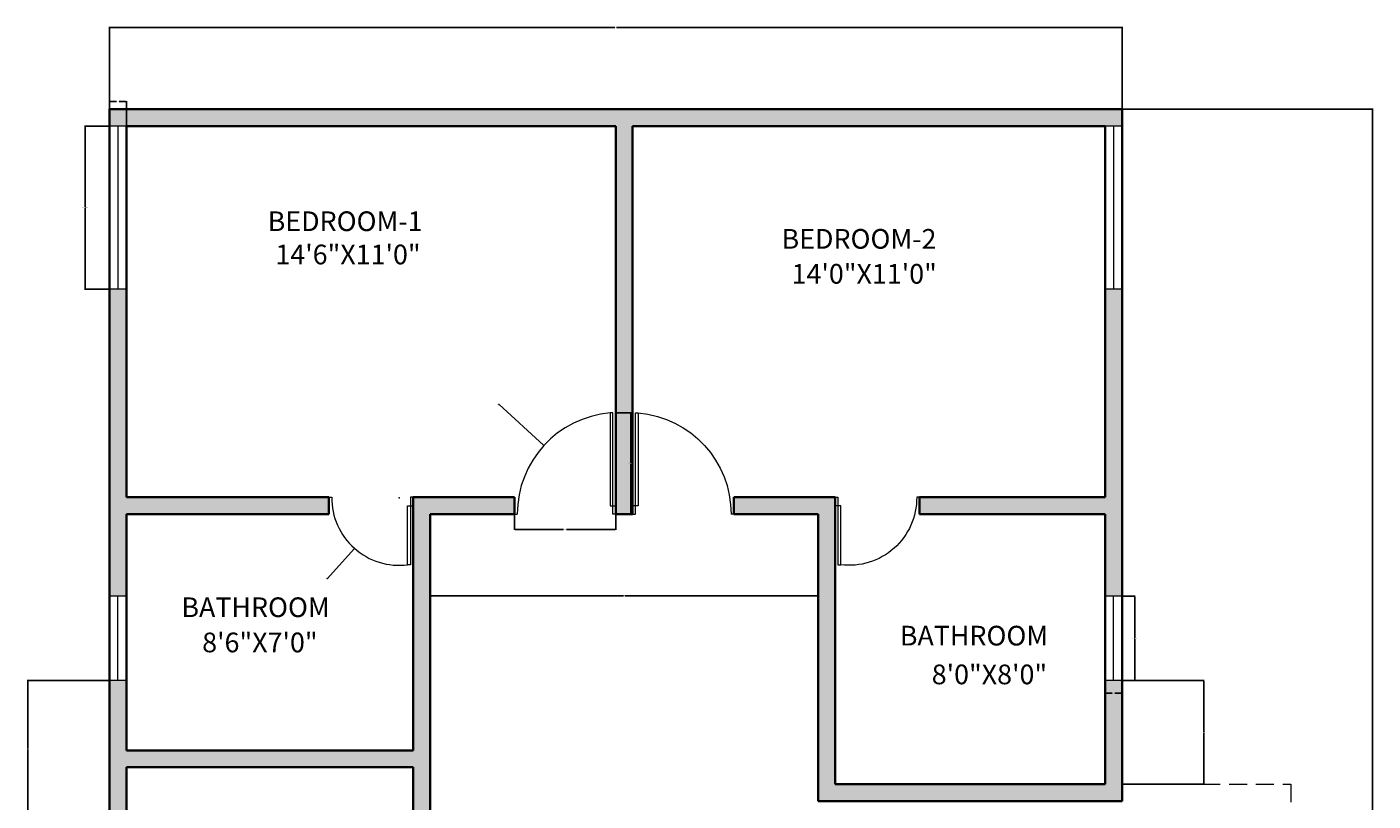
# Model space of a CAD drawing. Units: inches. Extents: x 2886 to 3365, y 1372 to 2008.
# Tile 2 of 2: x 2886 to 3365, y 1733 to 2008. Entities that reach past the tile are written whole.
import ezdxf

# ---------------------------------------------------------------- set-up
doc = ezdxf.new("R2010")
doc.units = ezdxf.units.IN
doc.linetypes.add('DASHED2', pattern=[9.525, 6.35, -3.175])
for name, color, linetype, lineweight in [('A-ANNO-DIMS', 2, 'Continuous', 18), ('A-AREA-IDEN', 50, 'Continuous', 18), ('A-DOOR', 230, 'Continuous', 18), ('A-FLOR-OVHD', 7, 'DASHED2', 18), ('A-GLAZ', 7, 'Continuous', 18), ('A-WALL', 7, 'Continuous', 35)]:
    doc.layers.add(name, color=color, linetype=linetype, lineweight=lineweight)
doc.layers.add('A-WALL-PATT', color=18, linetype='Continuous', lineweight=13, true_color=0x000000)
doc.styles.get("Standard").update_dxf_attribs({"font": 'arial.ttf'})
doc.dimstyles.get("Standard").update_dxf_attribs({"dimtxt": 0.18, "dimasz": 0.18, "dimexe": 0.18, "dimexo": 0.0625, "dimgap": 0.09, "dimtad": 0, "dimtih": 1, "dimtoh": 1, "dimdec": 4, "dimzin": 0, "dimdsep": 46, "dimtxsty": 'Standard', "dimcen": 0.09, "dimadec": 0, "dimazin": 0, "dimtfac": 1, "dimtdec": 4, "dimtofl": 0, "dimtmove": 0, "dimatfit": 3, "dimfxl": 1, "dimtolj": 1, "dimtzin": 0, "dimarcsym": 0})

# ---------------------------------------------------------------- blocks, each defined once
blk = doc.blocks.new('DOOR-SWING-30IN')
for p, q in [((0, 24.19), (1, 24.19)), ((30, 24.19), (29, 24.19)), ((29, 24.19), (29, 0.19)), ((28, 0.19), (28, 21.19)), ((28, 21.19), (30, 21.19)), ((29, 0.19), (28, 0.19))]:
    blk.add_line(p, q)
blk.add_arc((25, 24), 24, 179.5504, 277.1825)
blk = doc.blocks.new('DOOR-SWING-36IN')
for p, q in [((35, 36), (34, 36)), ((34, 36), (34, 3)), ((35, 0), (35, 36)), ((0, 0), (1, 0)), ((34, 3), (36, 3)), ((36, 0), (35, 0))]:
    blk.add_line(p, q)
blk.add_arc((37, 0.13), 36, 94.7798, 180.1993)
blk = doc.blocks.new('WIN-30IN')
for p, q in [((6, 30), (0, 30)), ((3, 0), (3, 30)), ((6, 0), (0, 0))]:
    blk.add_line(p, q)
blk = doc.blocks.new('WIN-58IN')
for p, q in [((6, 58), (0, 58)), ((3, 58), (3, 0)), ((6, 0), (0, 0))]:
    blk.add_line(p, q)
blk = doc.blocks.new('*D7')
at = {"layer": 'A-ANNO-DIMS', "color": 0, "lineweight": -2, "transparency": 16777216}
for p, q in [((3095.42, 1870.96), (3100.94, 1870.96)), ((3100.76, 1870.78), (3100.76, 1853.15)), ((3100.76, 1835.14), (3100.76, 1852.78)), ((3095.42, 1834.96), (3100.94, 1834.96))]:
    blk.add_line(p, q, dxfattribs=at)
at = {"layer": 'A-ANNO-DIMS', "color": 0, "transparency": 16777216}
for points in [[(3100.73, 1870.78), (3100.79, 1870.78), (3100.76, 1870.96)], [(3100.73, 1835.14), (3100.79, 1835.14), (3100.76, 1834.96)]]:
    blk.add_solid(points, dxfattribs=at)
at = {"layer": 'Defpoints', "color": 0, "transparency": 16777216}
for p in [(3095.36, 1870.96), (3100.76, 1870.96), (3095.36, 1834.96)]:
    blk.add_point(p, dxfattribs=at)
at = {"layer": 'A-ANNO-DIMS', "color": 0, "transparency": 16777216, "insert": (3100.76, 1852.96), "char_height": 0.18, "attachment_point": 5}
blk.add_mtext('\\A1;DOOR 36 TYP.', dxfattribs=at)
blk = doc.blocks.new('*D8')
at = {"layer": 'A-ANNO-DIMS', "color": 0, "lineweight": -2, "transparency": 16777216}
for p, q in [((3059.36, 1834.9), (3059.36, 1829.38)), ((3095.36, 1834.9), (3095.36, 1829.38)), ((3059.54, 1829.56), (3076.83, 1829.56)), ((3095.18, 1829.56), (3077.89, 1829.56))]:
    blk.add_line(p, q, dxfattribs=at)
at = {"layer": 'A-ANNO-DIMS', "color": 0, "transparency": 16777216}
for points in [[(3059.54, 1829.59), (3059.54, 1829.53), (3059.36, 1829.56)], [(3095.18, 1829.59), (3095.18, 1829.53), (3095.36, 1829.56)]]:
    blk.add_solid(points, dxfattribs=at)
at = {"layer": 'Defpoints', "color": 0, "transparency": 16777216}
for p in [(3059.36, 1834.96), (3095.36, 1834.96), (3095.36, 1829.56)]:
    blk.add_point(p, dxfattribs=at)
at = {"layer": 'A-ANNO-DIMS', "color": 0, "transparency": 16777216, "insert": (3077.36, 1829.56), "char_height": 0.18, "attachment_point": 5}
blk.add_mtext('\\A1;36 TYP.', dxfattribs=at)
blk = doc.blocks.new('*D9')
at = {"layer": 'A-ANNO-DIMS', "color": 0, "lineweight": -2, "transparency": 16777216}
for p, q in [((3275.42, 1805.81), (3280.04, 1805.81)), ((3279.86, 1805.63), (3279.86, 1790.99)), ((3279.86, 1775.99), (3279.86, 1790.63)), ((3275.42, 1775.81), (3280.04, 1775.81))]:
    blk.add_line(p, q, dxfattribs=at)
at = {"layer": 'A-ANNO-DIMS', "color": 0, "transparency": 16777216}
for points in [[(3279.83, 1805.63), (3279.89, 1805.63), (3279.86, 1805.81)], [(3279.83, 1775.99), (3279.89, 1775.99), (3279.86, 1775.81)]]:
    blk.add_solid(points, dxfattribs=at)
at = {"layer": 'Defpoints', "color": 0, "transparency": 16777216}
for p in [(3275.36, 1805.81), (3279.86, 1805.81), (3275.36, 1775.81)]:
    blk.add_point(p, dxfattribs=at)
at = {"layer": 'A-ANNO-DIMS', "color": 0, "transparency": 16777216, "insert": (3279.86, 1790.81), "char_height": 0.18, "attachment_point": 5}
blk.add_mtext('\\A1;WINDOW 30 TYP.', dxfattribs=at)
blk = doc.blocks.new('*D10')
at = {"layer": 'A-ANNO-DIMS', "color": 0, "lineweight": -2, "transparency": 16777216}
for p, q in [((3269.36, 1775.75), (3269.36, 1771.13)), ((3275.36, 1775.75), (3275.36, 1771.13)), ((3269.54, 1771.31), (3271.9, 1771.31)), ((3275.18, 1771.31), (3272.82, 1771.31))]:
    blk.add_line(p, q, dxfattribs=at)
at = {"layer": 'A-ANNO-DIMS', "color": 0, "transparency": 16777216}
for points in [[(3269.54, 1771.34), (3269.54, 1771.28), (3269.36, 1771.31)], [(3275.18, 1771.34), (3275.18, 1771.28), (3275.36, 1771.31)]]:
    blk.add_solid(points, dxfattribs=at)
at = {"layer": 'Defpoints', "color": 0, "transparency": 16777216}
for p in [(3269.36, 1775.81), (3275.36, 1775.81), (3275.36, 1771.31)]:
    blk.add_point(p, dxfattribs=at)
at = {"layer": 'A-ANNO-DIMS', "color": 0, "transparency": 16777216, "insert": (3272.36, 1771.31), "char_height": 0.18, "attachment_point": 5}
blk.add_mtext('\\A1;6 TYP.', dxfattribs=at)
blk = doc.blocks.new('*D11')
at = {"layer": 'A-ANNO-DIMS', "color": 0, "lineweight": -2, "transparency": 16777216}
for p, q in [((2915.29, 1972.96), (2906.48, 1972.96)), ((2906.66, 1972.78), (2906.66, 1944.15)), ((2906.66, 1915.14), (2906.66, 1943.78)), ((2915.29, 1914.96), (2906.48, 1914.96))]:
    blk.add_line(p, q, dxfattribs=at)
at = {"layer": 'A-ANNO-DIMS', "color": 0, "transparency": 16777216}
for points in [[(2906.63, 1972.78), (2906.69, 1972.78), (2906.66, 1972.96)], [(2906.63, 1915.14), (2906.69, 1915.14), (2906.66, 1914.96)]]:
    blk.add_solid(points, dxfattribs=at)
at = {"layer": 'Defpoints', "color": 0, "transparency": 16777216}
for p in [(2906.66, 1972.96), (2915.36, 1972.96), (2915.36, 1914.96)]:
    blk.add_point(p, dxfattribs=at)
at = {"layer": 'A-ANNO-DIMS', "color": 0, "transparency": 16777216, "insert": (2906.66, 1943.96), "char_height": 0.18, "attachment_point": 5}
blk.add_mtext('\\A1;WINDOW 58 TYP.', dxfattribs=at)
blk = doc.blocks.new('*D12')
at = {"layer": 'A-ANNO-DIMS', "color": 0, "lineweight": -2, "transparency": 16777216}
for p, q in [((2915.36, 1973.02), (2915.36, 1981.84)), ((2915.54, 1981.66), (2917.9, 1981.66)), ((2921.18, 1981.66), (2918.82, 1981.66)), ((2921.36, 1973.02), (2921.36, 1981.84))]:
    blk.add_line(p, q, dxfattribs=at)
at = {"layer": 'A-ANNO-DIMS', "color": 0, "transparency": 16777216}
for points in [[(2915.54, 1981.69), (2915.54, 1981.63), (2915.36, 1981.66)], [(2921.18, 1981.69), (2921.18, 1981.63), (2921.36, 1981.66)]]:
    blk.add_solid(points, dxfattribs=at)
at = {"layer": 'Defpoints', "color": 0, "transparency": 16777216}
for p in [(2921.36, 1981.66), (2915.36, 1972.96), (2921.36, 1972.96)]:
    blk.add_point(p, dxfattribs=at)
at = {"layer": 'A-ANNO-DIMS', "color": 0, "transparency": 16777216, "insert": (2918.36, 1981.66), "char_height": 0.18, "attachment_point": 5}
blk.add_mtext('\\A1;6 TYP.', dxfattribs=at)
blk = doc.blocks.new('*D14')
at = {"layer": 'A-ANNO-DIMS', "color": 0, "lineweight": -2, "transparency": 16777216}
for p, q in [((3275.42, 1978.96), (3364.59, 1978.96)), ((3364.41, 1978.78), (3364.41, 1690.14)), ((3364.41, 1401.14), (3364.41, 1689.78)), ((3275.42, 1400.96), (3364.59, 1400.96))]:
    blk.add_line(p, q, dxfattribs=at)
at = {"layer": 'A-ANNO-DIMS', "color": 0, "transparency": 16777216}
for points in [[(3364.38, 1978.78), (3364.44, 1978.78), (3364.41, 1978.96)], [(3364.38, 1401.14), (3364.44, 1401.14), (3364.41, 1400.96)]]:
    blk.add_solid(points, dxfattribs=at)
at = {"layer": 'Defpoints', "color": 0, "transparency": 16777216}
for p in [(3275.36, 1978.96), (3364.41, 1978.96), (3275.36, 1400.96)]:
    blk.add_point(p, dxfattribs=at)
at = {"layer": 'A-ANNO-DIMS', "color": 0, "transparency": 16777216, "insert": (3364.41, 1689.96), "char_height": 0.18, "attachment_point": 5}
blk.add_mtext('\\A1;578', dxfattribs=at)
blk = doc.blocks.new('*D15')
at = {"layer": 'A-ANNO-DIMS', "color": 0, "lineweight": -2, "transparency": 16777216}
for p, q in [((2915.36, 1979.02), (2915.36, 2008.19)), ((2915.54, 2008.01), (3095.07, 2008.01)), ((3275.18, 2008.01), (3095.65, 2008.01)), ((3275.36, 1979.02), (3275.36, 2008.19))]:
    blk.add_line(p, q, dxfattribs=at)
at = {"layer": 'A-ANNO-DIMS', "color": 0, "transparency": 16777216}
for points in [[(2915.54, 2008.04), (2915.54, 2007.98), (2915.36, 2008.01)], [(3275.18, 2008.04), (3275.18, 2007.98), (3275.36, 2008.01)]]:
    blk.add_solid(points, dxfattribs=at)
at = {"layer": 'Defpoints', "color": 0, "transparency": 16777216}
for p in [(3275.36, 2008.01), (2915.36, 1978.96), (3275.36, 1978.96)]:
    blk.add_point(p, dxfattribs=at)
at = {"layer": 'A-ANNO-DIMS', "color": 0, "transparency": 16777216, "insert": (3095.36, 2008.01), "char_height": 0.18, "attachment_point": 5}
blk.add_mtext('\\A1;360', dxfattribs=at)
blk = doc.blocks.new('*D20')
at = {"layer": 'A-ANNO-DIMS', "color": 0, "lineweight": -2, "transparency": 16777216}
for p, q in [((2915.29, 1775.81), (2886.13, 1775.81)), ((2886.31, 1775.63), (2886.31, 1751.69)), ((2886.31, 1727.38), (2886.31, 1751.32)), ((2915.29, 1727.2), (2886.13, 1727.2))]:
    blk.add_line(p, q, dxfattribs=at)
at = {"layer": 'A-ANNO-DIMS', "color": 0, "transparency": 16777216}
for points in [[(2886.28, 1775.63), (2886.34, 1775.63), (2886.31, 1775.81)], [(2886.28, 1727.38), (2886.34, 1727.38), (2886.31, 1727.2)]]:
    blk.add_solid(points, dxfattribs=at)
at = {"layer": 'Defpoints', "color": 0, "transparency": 16777216}
for p in [(2886.31, 1775.81), (2915.36, 1775.81), (2915.36, 1727.2)]:
    blk.add_point(p, dxfattribs=at)
at = {"layer": 'A-ANNO-DIMS', "color": 0, "transparency": 16777216, "insert": (2886.31, 1751.5), "char_height": 0.18, "attachment_point": 5}
blk.add_mtext('\\A1;48.61', dxfattribs=at)
blk = doc.blocks.new('*D23')
at = {"layer": 'A-ANNO-DIMS', "color": 0, "lineweight": -2, "transparency": 16777216}
for p, q in [((3275.42, 1775.81), (3304.59, 1775.81)), ((3304.41, 1775.63), (3304.41, 1757.57)), ((3304.41, 1739.14), (3304.41, 1757.2)), ((3275.42, 1738.96), (3304.59, 1738.96))]:
    blk.add_line(p, q, dxfattribs=at)
at = {"layer": 'A-ANNO-DIMS', "color": 0, "transparency": 16777216}
for points in [[(3304.38, 1775.63), (3304.44, 1775.63), (3304.41, 1775.81)], [(3304.38, 1739.14), (3304.44, 1739.14), (3304.41, 1738.96)]]:
    blk.add_solid(points, dxfattribs=at)
at = {"layer": 'Defpoints', "color": 0, "transparency": 16777216}
for p in [(3275.36, 1775.81), (3275.36, 1738.96), (3304.41, 1738.96)]:
    blk.add_point(p, dxfattribs=at)
at = {"layer": 'A-ANNO-DIMS', "color": 0, "transparency": 16777216, "insert": (3304.41, 1757.39), "char_height": 0.18, "attachment_point": 5}
blk.add_mtext('\\A1;36.85', dxfattribs=at)
blk = doc.blocks.new('*D25')
at = {"layer": 'A-ANNO-DIMS', "color": 0, "lineweight": -2, "transparency": 16777216}
for p, q in [((3029.36, 1834.9), (3029.36, 1805.73)), ((3167.36, 1834.9), (3167.36, 1805.73)), ((3029.54, 1805.91), (3098.08, 1805.91)), ((3167.18, 1805.91), (3098.64, 1805.91))]:
    blk.add_line(p, q, dxfattribs=at)
at = {"layer": 'A-ANNO-DIMS', "color": 0, "transparency": 16777216}
for points in [[(3029.54, 1805.94), (3029.54, 1805.88), (3029.36, 1805.91)], [(3167.18, 1805.94), (3167.18, 1805.88), (3167.36, 1805.91)]]:
    blk.add_solid(points, dxfattribs=at)
at = {"layer": 'Defpoints', "color": 0, "transparency": 16777216}
for p in [(3029.36, 1834.96), (3167.36, 1834.96), (3029.36, 1805.91)]:
    blk.add_point(p, dxfattribs=at)
at = {"layer": 'A-ANNO-DIMS', "color": 0, "transparency": 16777216, "insert": (3098.36, 1805.91), "char_height": 0.18, "attachment_point": 5}
blk.add_mtext('\\A1;138', dxfattribs=at)
blk = doc.blocks.new('*D31')
at = {"layer": 'A-ANNO-DIMS', "color": 0, "lineweight": -2, "transparency": 16777216}
for p, q in [((3053.72, 1874.01), (3053.9, 1874.01)), ((3053.9, 1874.01), (3069.69, 1859.54)), ((3096.27, 1835.09), (3096.45, 1835.09)), ((3096.36, 1835), (3096.36, 1835.18))]:
    blk.add_line(p, q, dxfattribs=at)
at = {"layer": 'A-ANNO-DIMS', "color": 0, "transparency": 16777216}
blk.add_solid([(3069.71, 1859.56), (3069.67, 1859.51), (3069.82, 1859.41)], dxfattribs=at)
at = {"layer": 'Defpoints', "color": 0, "transparency": 16777216}
for p in [(3069.82, 1859.41), (3096.36, 1835.09)]:
    blk.add_point(p, dxfattribs=at)
at = {"layer": 'A-ANNO-DIMS', "color": 0, "transparency": 16777216, "insert": (3053.41, 1874.01), "char_height": 0.18, "attachment_point": 5}
blk.add_mtext('\\A1;R36', dxfattribs=at)
blk = doc.blocks.new('*D32')
at = {"layer": 'A-ANNO-DIMS', "color": 0, "lineweight": -2, "transparency": 16777216}
for p, q in [((3018.27, 1840.77), (3018.45, 1840.77)), ((3018.36, 1840.68), (3018.36, 1840.86)), ((2992.85, 1812.07), (3002.29, 1822.7)), ((2992.67, 1812.07), (2992.85, 1812.07))]:
    blk.add_line(p, q, dxfattribs=at)
at = {"layer": 'A-ANNO-DIMS', "color": 0, "transparency": 16777216}
blk.add_solid([(3002.27, 1822.72), (3002.31, 1822.68), (3002.41, 1822.84)], dxfattribs=at)
at = {"layer": 'Defpoints', "color": 0, "transparency": 16777216}
for p in [(3018.36, 1840.77), (3002.41, 1822.84)]:
    blk.add_point(p, dxfattribs=at)
at = {"layer": 'A-ANNO-DIMS', "color": 0, "transparency": 16777216, "insert": (2992.17, 1812.07), "char_height": 0.18, "attachment_point": 5}
blk.add_mtext('\\A1;3X R24', dxfattribs=at)

msp = doc.modelspace()

# ---------------------------------------------------------------- hatches: boundary and pattern name
at = {"layer": 'A-WALL-PATT'}
h = msp.add_hatch(color=256, dxfattribs=at)
h.dxf.hatch_style = 1
h.paths.add_polyline_path([(3275.3575, 1978.9624), (2915.3575, 1978.9624), (2915.3575, 1972.9624), (2921.3575, 1972.9624), (3095.3575, 1972.9624), (3095.3575, 1834.9624), (3101.3575, 1834.9624), (3101.3575, 1972.9624), (3269.3575, 1972.9624), (3275.3575, 1972.9624)])
h = msp.add_hatch(color=256, dxfattribs=at)
h.dxf.hatch_style = 1
h.paths.add_polyline_path([(2993.3575, 1840.9624), (2921.3575, 1840.9624), (2921.3575, 1914.9624), (2915.3575, 1914.9624), (2915.3575, 1805.8094), (2921.3575, 1805.8094), (2921.3575, 1834.9624), (2993.3575, 1834.9624)])
h = msp.add_hatch(color=256, dxfattribs=at)
h.dxf.hatch_style = 1
h.paths.add_polyline_path([(3275.3575, 1914.9624), (3269.3575, 1914.9624), (3269.3575, 1840.9624), (3203.3575, 1840.9624), (3203.3575, 1834.9624), (3269.3575, 1834.9624), (3269.3575, 1805.8094), (3275.3575, 1805.8094)])
h = msp.add_hatch(color=256, dxfattribs=at)
h.dxf.hatch_style = 1
h.paths.add_polyline_path([(3059.3575, 1840.9624), (3023.3575, 1840.9624), (3023.3575, 1750.9624), (2921.3575, 1750.9624), (2921.3575, 1775.8094), (2915.3575, 1775.8094), (2915.3575, 1727.2), (2921.3575, 1727.2), (2921.3575, 1744.9624), (3023.3575, 1744.9624), (3023.3575, 1666.9624), (3029.3575, 1666.9624), (3029.3575, 1834.9624), (3059.3575, 1834.9624)])
h = msp.add_hatch(color=256, dxfattribs=at)
h.dxf.hatch_style = 1
h.paths.add_polyline_path([(3173.3575, 1840.9624), (3137.3575, 1840.9624), (3137.3575, 1834.9624), (3167.3575, 1834.9624), (3167.3575, 1732.9624), (3275.3575, 1732.9624), (3275.3575, 1775.8094), (3269.3575, 1775.8094), (3269.3575, 1738.9624), (3173.3575, 1738.9624)])

# ---------------------------------------------------------------- linework, layer by layer
at = {"layer": 'A-FLOR-OVHD'}
for p, q in [((3275.3575, 1738.9624), (3335.3575, 1738.9624)), ((3335.3575, 1738.9624), (3335.3575, 1627.9624))]:
    msp.add_line(p, q, dxfattribs=at)
at = {"layer": 'A-WALL'}
for p, q in [((2921.3575, 1972.9624), (3095.3575, 1972.9624)), ((2921.3575, 1840.9624), (2921.3575, 1972.9624)), ((3095.3575, 1834.9624), (3095.3575, 1972.9624)), ((3101.3575, 1834.9624), (3101.3575, 1972.9624)), ((3101.3575, 1972.9624), (3269.3575, 1972.9624)), ((3269.3575, 1972.9624), (3269.3575, 1840.9624)), ((2921.3575, 1840.9624), (2993.3575, 1840.9624)), ((2993.3575, 1834.9624), (2993.3575, 1840.9624)), ((3023.3575, 1750.9624), (3023.3575, 1840.9624)), ((3023.3575, 1840.9624), (3059.3575, 1840.9624)), ((3059.3575, 1834.9624), (3059.3575, 1840.9624)), ((3137.3575, 1840.9624), (3173.3575, 1840.9624)), ((3137.3575, 1834.9624), (3137.3575, 1840.9624)), ((3173.3575, 1840.9624), (3173.3575, 1738.9624)), ((3203.3575, 1840.9624), (3203.3575, 1834.9624)), ((3203.3575, 1840.9624), (3269.3575, 1840.9624)), ((2921.3575, 1834.9624), (2993.3575, 1834.9624)), ((2921.3575, 1750.9624), (2921.3575, 1834.9624)), ((3029.3575, 1666.9624), (3029.3575, 1834.9624)), ((3029.3575, 1834.9624), (3059.3575, 1834.9624)), ((3095.3575, 1834.9624), (3101.3575, 1834.9624)), ((3137.3575, 1834.9624), (3167.3575, 1834.9624)), ((3167.3575, 1834.9624), (3167.3575, 1732.9624)), ((3203.3575, 1834.9624), (3269.3575, 1834.9624)), ((3269.3575, 1834.9624), (3269.3575, 1738.9624)), ((2921.3575, 1750.9624), (3023.3575, 1750.9624)), ((2921.3575, 1744.9624), (3023.3575, 1744.9624)), ((2921.3575, 1672.9624), (2921.3575, 1744.9624)), ((3023.3575, 1666.9624), (3023.3575, 1744.9624)), ((3173.3575, 1738.9624), (3269.3575, 1738.9624)), ((3167.3575, 1732.9624), (3275.3575, 1732.9624))]:
    msp.add_line(p, q, dxfattribs=at)
msp.add_lwpolyline([(3149.3575, 1400.9624), (2915.3575, 1400.9624), (2915.3575, 1978.9624), (3275.3575, 1978.9624), (3275.3575, 1732.9624)], dxfattribs=at)

# ---------------------------------------------------------------- block references
at = {"layer": 'A-DOOR'}
for name, p in [('DOOR-SWING-36IN', (3059.357, 1834.962)), ('DOOR-SWING-30IN', (2993.357, 1816.775))]:
    msp.add_blockref(name, p, dxfattribs=at)
at = {"layer": 'A-DOOR', "extrusion": (0, 0, -1), "zscale": -1}
for name, p in [('DOOR-SWING-36IN', (-3137.358, 1834.962)), ('DOOR-SWING-30IN', (-3203.358, 1816.775))]:
    msp.add_blockref(name, p, dxfattribs=at)
at = {"layer": 'A-GLAZ'}
for name, p in [('WIN-58IN', (2915.357, 1914.962)), ('WIN-58IN', (3269.357, 1914.962)), ('WIN-30IN', (2915.357, 1775.809)), ('WIN-30IN', (3269.357, 1775.809))]:
    msp.add_blockref(name, p, dxfattribs=at)

# ---------------------------------------------------------------- texts
at = {"layer": 'A-AREA-IDEN'}
for tag, p in [('BEDROOM-1', (2971.59, 1935.6085)), ('BEDROOM-2', (3154.297, 1929.3448)), ('14\'6"X11\'0"', (2974.3448, 1923.7918)), ('14\'0"X11\'0"', (3157.8713, 1916.9161)), ('BATHROOM', (2940.9158, 1798.3669)), ('BATHROOM', (3196.3511, 1788.2757)), ('8\'6"X7\'0"', (2948.3114, 1785.862)), ('8\'0"X8\'0"', (3207.6925, 1774.494))]:
    msp.add_attdef(tag, p, '', height=7, dxfattribs=at)

# ---------------------------------------------------------------- dimensions: what is measured, and where the dimension line sits
at = {"layer": 'A-ANNO-DIMS'}
dim = msp.add_linear_dim(base=(3275.3575, 2008.0124), p1=(2915.3575, 1978.9624), p2=(3275.3575, 1978.9624), dimstyle='Standard', override={"dimdec": 0, "dimlfac": 1, "dimrnd": 0, "dimzin": 0, "dimdsep": 46, "dimlunit": 2}, dxfattribs=at)
dim.commit()
dim.dimension.update_dxf_attribs({"geometry": '*D15', "text_midpoint": (3095.3575, 2008.0124)})
for base, p1, p2, picture, middle in [((2921.3575, 1981.6624), (2915.3575, 1972.9624), (2921.3575, 1972.9624), '*D12', (2918.3575, 1981.6624)), ((3095.3575, 1829.5624), (3059.3575, 1834.9624), (3095.3575, 1834.9624), '*D8', (3077.3575, 1829.5624)), ((3275.3575, 1771.3094), (3269.3575, 1775.8094), (3275.3575, 1775.8094), '*D10', (3272.3575, 1771.3094))]:
    dim = msp.add_linear_dim(base=base, p1=p1, p2=p2, text='<> TYP.', dimstyle='Standard', override={"dimdec": 0, "dimlfac": 1, "dimrnd": 0, "dimzin": 0, "dimdsep": 46, "dimlunit": 2}, dxfattribs=at)
    dim.commit()
    dim.dimension.update_dxf_attribs({"geometry": picture, "text_midpoint": middle})
for base, p1, p2, angle, override, picture, middle in [((3364.4075, 1978.9624), (3275.3575, 1400.9624), (3275.3575, 1978.9624), 90, {"dimdec": 0, "dimlfac": 1, "dimrnd": 0, "dimzin": 0, "dimdsep": 46, "dimlunit": 2}, '*D14', (3364.4075, 1689.9624)), ((3029.3575, 1805.9124), (3167.3575, 1834.9624), (3029.3575, 1834.9624), 180, {"dimdec": 0, "dimlfac": 1, "dimrnd": 0, "dimzin": 0, "dimdsep": 46, "dimlunit": 2}, '*D25', (3098.3575, 1805.9124)), ((2886.3075, 1775.8094), (2915.3575, 1727.2), (2915.3575, 1775.8094), 90, {"dimdec": 2, "dimlfac": 1, "dimrnd": 0, "dimzin": 0, "dimdsep": 46, "dimlunit": 2}, '*D20', (2886.3075, 1751.5047)), ((3304.4075, 1738.9624), (3275.3575, 1775.8094), (3275.3575, 1738.9624), 270, {"dimdec": 2, "dimlfac": 1, "dimrnd": 0, "dimzin": 0, "dimdsep": 46, "dimlunit": 2}, '*D23', (3304.4075, 1757.3859))]:
    dim = msp.add_linear_dim(base=base, p1=p1, p2=p2, angle=angle, dimstyle='Standard', override=override, dxfattribs=at)
    dim.commit()
    dim.dimension.update_dxf_attribs({"geometry": picture, "text_midpoint": middle})
for base, p1, p2, text, picture, middle in [((2906.6575, 1972.9624), (2915.3575, 1914.9624), (2915.3575, 1972.9624), 'WINDOW <> TYP.', '*D11', (2906.6575, 1943.9624)), ((3100.7575, 1870.9624), (3095.3575, 1834.9624), (3095.3575, 1870.9624), 'DOOR <> TYP.', '*D7', (3100.7575, 1852.9624)), ((3279.8575, 1805.8094), (3275.3575, 1775.8094), (3275.3575, 1805.8094), 'WINDOW <> TYP.', '*D9', (3279.8575, 1790.8094))]:
    dim = msp.add_linear_dim(base=base, p1=p1, p2=p2, angle=90, text=text, dimstyle='Standard', override={"dimdec": 0, "dimlfac": 1, "dimrnd": 0, "dimzin": 0, "dimdsep": 46, "dimlunit": 2}, dxfattribs=at)
    dim.commit()
    dim.dimension.update_dxf_attribs({"geometry": picture, "text_midpoint": middle})
dim = msp.add_radius_dim(center=(3096.3573, 1835.0876), mpoint=(3069.82, 1859.414), dimstyle='Standard', override={"dimdec": 0, "dimlfac": 1, "dimrnd": 0, "dimzin": 0, "dimdsep": 46, "dimlunit": 2}, dxfattribs=at)
dim.commit()
dim.dimension.update_dxf_attribs({"geometry": '*D31', "text_midpoint": (3053.4126, 1874.0098), "dimtype": 164})
dim = msp.add_radius_dim(center=(3018.3568, 1840.7741), mpoint=(3002.4121, 1822.8362), text='3X <>', dimstyle='Standard', override={"dimdec": 0, "dimlfac": 1, "dimrnd": 0, "dimzin": 0, "dimdsep": 46, "dimlunit": 2}, dxfattribs=at)
dim.commit()
dim.dimension.update_dxf_attribs({"geometry": '*D32', "text_midpoint": (2992.1674, 1812.0734), "dimtype": 164})

doc.saveas('drawing.dxf')
